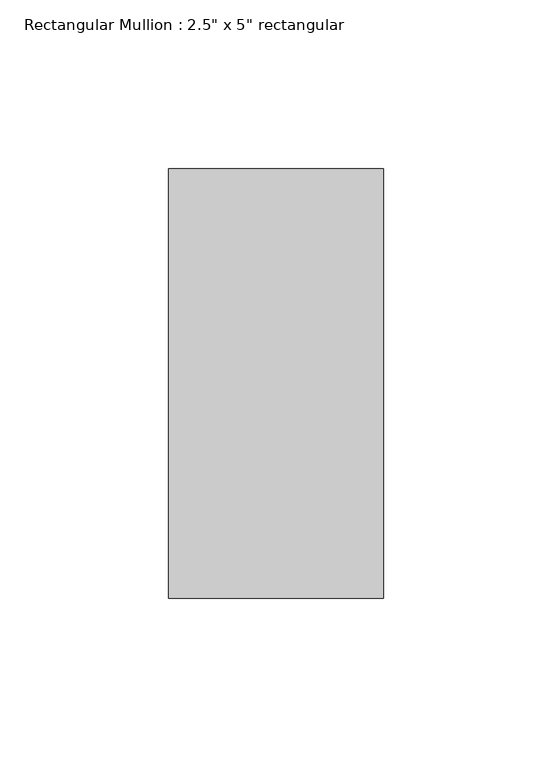
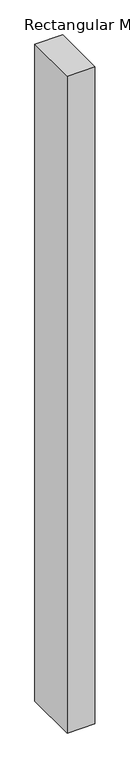
"""IFC4 building model written with IfcOpenShell, lengths in millimetres: member geometry."""

from ifc_helpers import new_model, si_unit, frame, origin, place, context, project, spatial, polyline, outline, extrude, source, transform, mapped, element, save


def member_b4cb8141(model_context):
    return source(origin(), model_context, "Body", "SweptSolid", [
        extrude(outline(polyline([(0.0, 63.5), (0.0, -63.5), (-63.5, -63.5), (-63.5, 63.5), (0.0, 63.5)])), frame((0.0, 0.0, -1586.1267095), z_axis=(0.0, 0.0, 1.0), x_axis=(1.0, 0.0, 0.0)), (0.0, 0.0, 1.0), 1586.1267095),
    ])


if __name__ == "__main__":
    model = new_model("IFC4")
    model_context = context("Model", 3, world=origin())
    ifc_project = project(units=[si_unit("LENGTHUNIT", "METRE", prefix="MILLI")], contexts=[model_context])
    site = spatial("IfcSite", under=ifc_project)
    building = spatial("IfcBuilding", under=site)
    placement = place(None, origin())
    member_shape = member_b4cb8141(model_context)
    element("IfcMember", 1, ObjectType="Rectangular Mullion : 2.5\" x 5\" rectangular", at=placement, inside=building, context=model_context, shape_type="MappedRepresentation", body=[
        mapped(member_shape, transform((0.0, 0.0, 0.0), x_axis=(1.0, 0.0, 0.0), y_axis=(0.0, 1.0, 0.0), z_axis=(0.0, 0.0, 1.0))),
    ])
    save(model, "model.ifc")

# Revit data of these elements
# Type "Rectangular Mullion : 2.5\" x 5\" rectangular"
#   built-in parameter 1007304 = 0.416667 (stored number, unit not read)
#   built-in parameter 1007301 = 0.104167 (stored number, unit not read)
#   built-in parameter 1007300 = 0.104167 (stored number, unit not read)
# Element 1 (IfcMember, "Rectangular Mullion : 2.5\" x 5\" rectangular")
#   Materials on its faces: "Aluminum"
# Materials
#   "Aluminum": class "Metal", colour RGB 247 247 247, transparency 0, Description = "Aluminum 6061", Cost = 0
